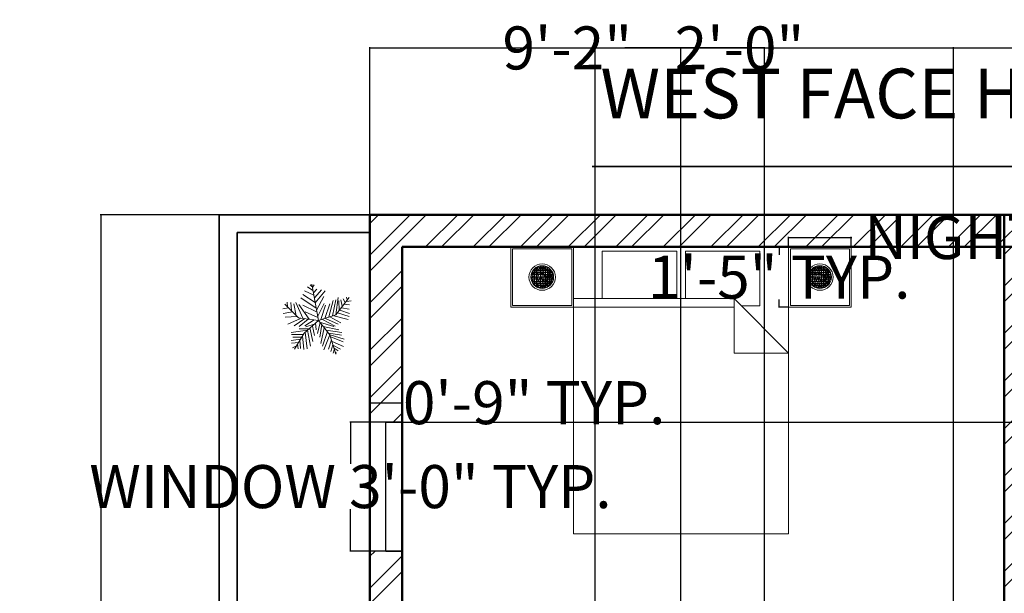
# Model space of a CAD drawing. Units: inches. Extents: x -40 to 578, y -482 to 237.
# Tile 5 of 7: x -26 to 249, y 67 to 227. Entities that reach past the tile are written whole.
import ezdxf

# ---------------------------------------------------------------- set-up
doc = ezdxf.new("R2010")
doc.units = ezdxf.units.IN
doc.header["$MEASUREMENT"] = 0
for name, color, linetype, lineweight in [('A-ANNO-DIMS', 2, 'Continuous', 18), ('A-ANNO-TEXT', 7, 'Continuous', 35), ('A-FURN', 4, 'Continuous', 18), ('A-WALL-PATT', 252, 'Continuous', 13), ('C-PROP', 3, 'Continuous', 35), ('L-PLNT', 94, 'Continuous', 13), ('WALLS', 3, 'Continuous', 50), ('WINDOWS', 241, 'Continuous', 25)]:
    doc.layers.add(name, color=color, linetype=linetype, lineweight=lineweight)
doc.styles.get("Standard").update_dxf_attribs({"font": 'arial.ttf'})
doc.dimstyles.get("Standard").update_dxf_attribs({"dimtxt": 12, "dimasz": 0.18, "dimexe": 0.18, "dimexo": 0.0625, "dimgap": 0.09, "dimtad": 0, "dimtih": 1, "dimtoh": 1, "dimdec": 0, "dimzin": 0, "dimdsep": 46, "dimlunit": 3, "dimtxsty": 'Standard', "dimcen": 0.09, "dimadec": 0, "dimazin": 0, "dimtfac": 1, "dimtdec": 0, "dimtofl": 0, "dimtmove": 0, "dimatfit": 3, "dimfxl": 1, "dimtolj": 1, "dimtzin": 0, "dimarcsym": 0})

# ---------------------------------------------------------------- blocks, each defined once
blk = doc.blocks.new('Bed - Queen')
for p, q in [((0, -80.00003), (0, 0)), ((0, 0), (59.99999, 0)), ((59.99999, 0), (59.99999, -80.00003)), ((7.99999, -1.2), (28.79998, -1.2)), ((7.99999, -14.4), (7.99999, -1.2)), ((28.79998, -1.2), (28.79998, -14.4)), ((31.19999, -1.2), (51.99999, -1.2)), ((31.19999, -14.4), (31.19999, -1.2)), ((51.99999, -1.2), (51.99999, -16.4)), ((0, -14.4), (44.8, -14.4)), ((59.99999, -29.6), (44.8, -14.4)), ((44.8, -14.4), (44.8, -29.6)), ((51.99999, -16.4), (46.79936, -16.4)), ((44.8, -16.8), (0, -16.8)), ((44.8, -29.6), (59.99999, -29.6)), ((59.99999, -80.00003), (0, -80.00003))]:
    blk.add_line(p, q)
blk = doc.blocks.new('*U14')
for p, q in [((-185.1152, 1008.5578), (-553.1612, 1185.4942)), ((-221.9198, 1197.3052), (-433.5526, 1338.8594)), ((-258.7244, 1362.456), (-332.3336, 1421.4348)), ((0, 0), (-266.7, 1447.8)), ((-231.1146, 1315.2628), (-166.7002, 1421.4348)), ((-194.31, 1102.9442), (-65.4812, 1256.284)), ((-148.3106, 914.1968), (118.5418, 1220.9018)), ((-129.8956, 701.8528), (265.7602, 1185.4942)), ((-93.091, 489.5342), (-700.3796, 902.3858)), ((-129.8956, 713.6638), (-626.7704, 1032.1544)), ((-74.7014, 418.7444), (219.7608, 961.39)), ((412.9786, 147.447), (587.8068, 796.2392)), ((560.197, 182.8292), (698.2206, 819.8358)), ((685.8, 228.6), (1219.2, 914.4)), ((689.0258, 230.0224), (790.2448, 914.1968)), ((891.4384, 831.6214), (946.658, 572.1096)), ((983.4626, 867.0036), (1066.2666, 725.4494)), ((1121.4862, 925.9824), (1149.0706, 831.6214)), ((-1206.4492, 501.3198), (-1418.082, 465.9376)), ((-800.1, 114.3), (-1333.5, 647.7)), ((-1234.059, 536.7274), (-1252.4486, 737.2604)), ((-1105.2302, 725.4494), (-1077.6458, 395.1732)), ((-976.4268, 666.4706), (-884.4026, 194.6402)), ((-902.8176, 713.6638), (-617.5756, 100.2538)), ((-369.1382, 53.086), (-783.1836, 642.874)), ((-617.5756, 607.4918), (-74.7014, 347.98)), ((-28.6766, 171.0436), (228.9556, 678.2816)), ((100.1268, 41.275), (284.1498, 619.2774)), ((256.5654, 88.4682), (449.7832, 666.4706)), ((808.6344, 784.4282), (827.0494, 418.7444)), ((845.439, 418.7444), (1241.0948, 277.1902)), ((919.0482, 501.3198), (1222.6798, 454.152)), ((1029.462, 654.685), (1241.0948, 631.0884)), ((1112.2914, 760.8316), (1296.3144, 784.4282)), ((-1031.621, 347.98), (-1399.667, 277.1902)), ((-847.598, 159.2326), (-1326.0578, 135.636)), ((-718.7946, 88.4682), (-1215.644, -147.447)), ((-543.9664, 76.6572), (-967.2066, -206.4512)), ((0, 0), (-800.1, 114.3)), ((-405.9428, 53.086), (-764.794, -241.8334)), ((0, 0), (-571.5, -495.3)), ((-166.7002, 29.4894), (-543.9664, -206.4512)), ((-525.5514, 347.98), (-28.6766, 123.8504)), ((0, 0), (685.8, 228.6)), ((0, 0), (457.2, -571.5)), ((164.5412, 41.275), (661.416, -218.2368)), ((284.1498, 88.4682), (781.0246, -147.447)), ((458.978, 147.447), (891.4384, -88.4682)), ((615.4166, 194.6402), (1185.8752, 41.275)), ((753.4148, 312.5978), (1222.6798, 159.2326)), ((-442.7474, -383.3876), (-1086.8406, -477.7486)), ((-387.5278, -324.4088), (-764.794, -324.4088)), ((-166.7002, -147.447), (-507.1618, -253.619)), ((-433.5526, -383.3876), (-323.1134, -1020.3688)), ((-341.5284, -289.0012), (-221.9198, -831.6214)), ((-240.3094, -218.2368), (-157.5054, -595.7062)), ((-120.7008, -88.4682), (-93.091, -371.5766)), ((63.3222, -76.6826), (-37.8714, -513.1308)), ((44.9326, -64.897), (615.4166, -241.8334)), ((127.7366, -159.258), (54.1274, -654.685)), ((228.9556, -289.0012), (90.932, -914.1968)), ((192.151, -230.0224), (817.8292, -371.5766)), ((311.7596, -383.3876), (937.4378, -477.7486)), ((-718.7946, -737.2604), (-1086.8406, -796.2392)), ((-617.5756, -548.5384), (-1077.6458, -560.324)), ((-681.9646, -666.496), (-1022.4262, -654.685)), ((-571.5, -495.3), (-952.5, -1143)), ((-737.1842, -784.4536), (-709.5744, -1114.7298)), ((-635.9652, -607.5172), (-580.771, -1150.1374)), ((-525.5514, -465.963), (-451.9422, -1126.5408)), ((357.759, -430.5554), (164.5412, -1020.3688)), ((458.978, -572.1096), (210.5406, -1161.923)), ((514.1976, -772.6426), (403.7838, -1138.3264)), ((412.9786, -501.3452), (919.0482, -583.9206)), ((457.2, -571.5), (685.8, -1333.5)), ((468.1982, -572.1096), (1029.462, -737.2604)), ((486.5878, -642.8994), (983.4626, -843.4324)), ((-783.1836, -867.029), (-1077.6458, -902.4112)), ((-875.2078, -1008.5832), (-1040.8412, -1079.3476)), ((-829.2084, -937.7934), (-810.7934, -1126.5408)), ((578.612, -961.39), (495.7826, -1232.7128)), ((541.8074, -831.6214), (992.6574, -1032.1544)), ((578.612, -973.1756), (873.0488, -1138.3264)), ((624.6114, -1161.923), (587.8068, -1291.6916)), ((624.6114, -1102.9442), (781.0246, -1209.1162)), ((679.8056, -1268.095), (716.6102, -1291.6916))]:
    blk.add_line(p, q)
blk = doc.blocks.new('NIGHTSTAND-LAMP')
for p, q in [((7.17, 11.17), (5.64, 7.78)), ((7.58, 11.36), (5.82, 7.16)), ((8.24, 11.54), (6.14, 6.59)), ((8.75, 11.58), (6.65, 6.01)), ((9.21, 11.55), (7.17, 5.63)), ((7.17, 11.17), (10.32, 11.17)), ((7.17, 11.17), (7.17, 5.63)), ((9.71, 11.43), (7.58, 5.44)), ((7.58, 11.36), (7.58, 5.44)), ((8.24, 11.54), (8.24, 5.18)), ((10.22, 11.22), (8.24, 5.26)), ((8.75, 11.58), (8.75, 5.22)), ((9.21, 11.55), (9.21, 5.18)), ((9.71, 11.43), (9.71, 5.37)), ((10.22, 11.22), (10.22, 5.58)), ((6.65, 10.79), (5.56, 8.46)), ((5.56, 8.4), (11.93, 8.4)), ((6.14, 10.22), (5.64, 9.09)), ((5.64, 9.09), (11.85, 9.09)), ((5.64, 9.09), (5.64, 7.71)), ((5.83, 9.68), (11.66, 9.68)), ((6.14, 10.22), (11.36, 10.22)), ((6.14, 10.22), (6.14, 6.58)), ((6.5, 10.65), (10.99, 10.65)), ((6.65, 10.79), (6.65, 6.01)), ((10.75, 10.87), (8.75, 5.22)), ((10.99, 10.65), (9.21, 5.18)), ((11.15, 10.48), (9.71, 5.37)), ((11.36, 10.22), (10.22, 5.58)), ((10.75, 10.87), (10.75, 5.93)), ((11.66, 9.68), (10.75, 5.93)), ((11.15, 10.48), (11.15, 6.31)), ((11.85, 9.09), (11.15, 6.31)), ((11.81, 9.26), (11.81, 7.54)), ((5.63, 7.78), (11.87, 7.78)), ((5.82, 7.16), (11.68, 7.16)), ((6.13, 6.59), (11.37, 6.59)), ((6.6, 6.05), (10.9, 6.05)), ((7.18, 5.63), (10.31, 5.63))]:
    blk.add_line(p, q)
for points in [[(17.49, 16.8), (0, 16.8), (0, 0), (17.49, 0)], [(16.99, 16.3), (0.5, 16.3), (0.5, 0.5), (16.99, 0.5)]]:
    blk.add_lwpolyline(points, close=True)
for radius in [3.68, 3.18]:
    blk.add_circle((8.75, 8.4), radius)
blk = doc.blocks.new('WIN-36IN')
for p, q in [((9, 36), (0, 36)), ((4.5, 0), (4.5, 36)), ((4.5, 36), (9, 36)), ((9, 0), (0, 0)), ((4.5, 0), (9, 0))]:
    blk.add_line(p, q)
blk = doc.blocks.new('*D26')
at = {"layer": 'A-ANNO-DIMS', "color": 0, "lineweight": -2, "transparency": 16777216}
for p, q in [((71.68, 114.63), (66.16, 114.63)), ((66.34, 114.45), (66.34, 102.94)), ((66.34, 78.81), (66.34, 90.33)), ((71.68, 78.63), (66.16, 78.63))]:
    blk.add_line(p, q, dxfattribs=at)
at = {"layer": 'A-ANNO-DIMS', "color": 0, "transparency": 16777216}
for points in [[(66.31, 114.45), (66.37, 114.45), (66.34, 114.63)], [(66.31, 78.81), (66.37, 78.81), (66.34, 78.63)]]:
    blk.add_solid(points, dxfattribs=at)
at = {"layer": 'Defpoints', "color": 0, "transparency": 16777216}
for p in [(66.34, 114.63), (71.74, 114.63), (71.74, 78.63)]:
    blk.add_point(p, dxfattribs=at)
at = {"layer": 'A-ANNO-DIMS', "color": 0, "transparency": 16777216, "insert": (66.34, 96.63), "char_height": 12, "attachment_point": 5}
blk.add_mtext('\\A1;WINDOW 3\'-0" TYP.', dxfattribs=at)
blk = doc.blocks.new('*D27')
at = {"layer": 'A-ANNO-DIMS', "color": 0, "lineweight": -2, "transparency": 16777216}
for p, q in [((71.74, 114.7), (71.74, 120.21)), ((71.92, 120.03), (80.56, 120.03)), ((80.74, 114.7), (80.74, 120.21)), ((80.74, 120.03), (80.92, 120.03))]:
    blk.add_line(p, q, dxfattribs=at)
at = {"layer": 'A-ANNO-DIMS', "color": 0, "transparency": 16777216}
for points in [[(71.92, 120.06), (71.92, 120), (71.74, 120.03)], [(80.56, 120.06), (80.56, 120), (80.74, 120.03)]]:
    blk.add_solid(points, dxfattribs=at)
at = {"layer": 'Defpoints', "color": 0, "transparency": 16777216}
for p in [(80.74, 120.03), (71.74, 114.63), (80.74, 114.63)]:
    blk.add_point(p, dxfattribs=at)
at = {"layer": 'A-ANNO-DIMS', "color": 0, "transparency": 16777216, "insert": (117.58, 120.03), "char_height": 12, "attachment_point": 5}
blk.add_mtext('\\A1;0\'-9" TYP.', dxfattribs=at)
blk = doc.blocks.new('*D28')
at = {"layer": 'A-ANNO-DIMS', "color": 0, "lineweight": -2, "transparency": 16777216}
for p, q in [((188.56, 163.51), (188.56, 166.25)), ((188.74, 166.07), (205.87, 166.07)), ((206.05, 163.51), (206.05, 166.25)), ((206.05, 166.07), (206.23, 166.07))]:
    blk.add_line(p, q, dxfattribs=at)
at = {"layer": 'A-ANNO-DIMS', "color": 0, "transparency": 16777216}
for points in [[(188.74, 166.1), (188.74, 166.04), (188.56, 166.07)], [(205.87, 166.1), (205.87, 166.04), (206.05, 166.07)]]:
    blk.add_solid(points, dxfattribs=at)
at = {"layer": 'Defpoints', "color": 0, "transparency": 16777216}
for p in [(206.05, 166.07), (188.56, 163.45), (206.05, 163.45)]:
    blk.add_point(p, dxfattribs=at)
at = {"layer": 'A-ANNO-DIMS', "color": 0, "transparency": 16777216, "insert": (313.4, 166.07), "char_height": 12, "attachment_point": 5}
blk.add_mtext('\\A1;NIGHTSTAND 1\'-5 1/2" TYP.', dxfattribs=at)
blk = doc.blocks.new('*D29')
at = {"layer": 'A-ANNO-DIMS', "color": 0, "lineweight": -2, "transparency": 16777216}
for p, q in [((188.5, 163.45), (185.76, 163.45)), ((185.94, 163.27), (185.94, 161.26)), ((185.94, 146.83), (185.94, 148.83)), ((188.5, 146.65), (185.76, 146.65))]:
    blk.add_line(p, q, dxfattribs=at)
at = {"layer": 'A-ANNO-DIMS', "color": 0, "transparency": 16777216}
for points in [[(185.91, 163.27), (185.97, 163.27), (185.94, 163.45)], [(185.91, 146.83), (185.97, 146.83), (185.94, 146.65)]]:
    blk.add_solid(points, dxfattribs=at)
at = {"layer": 'Defpoints', "color": 0, "transparency": 16777216}
for p in [(185.94, 163.45), (188.56, 163.45), (188.56, 146.65)]:
    blk.add_point(p, dxfattribs=at)
at = {"layer": 'A-ANNO-DIMS', "color": 0, "transparency": 16777216, "insert": (185.94, 155.05), "char_height": 12, "attachment_point": 5}
blk.add_mtext('\\A1;1\'-5" TYP.', dxfattribs=at)
blk = doc.blocks.new('*D42')
at = {"layer": 'A-ANNO-DIMS', "color": 0, "lineweight": -2, "transparency": 16777216}
for p, q in [((71.78, -441.49), (71.78, 219.12)), ((71.96, 218.94), (110.77, 218.94)), ((181.65, 218.94), (142.84, 218.94)), ((181.83, -441.49), (181.83, 219.12))]:
    blk.add_line(p, q, dxfattribs=at)
at = {"layer": 'A-ANNO-DIMS', "color": 0, "transparency": 16777216}
for points in [[(71.96, 218.97), (71.96, 218.91), (71.78, 218.94)], [(181.65, 218.97), (181.65, 218.91), (181.83, 218.94)]]:
    blk.add_solid(points, dxfattribs=at)
at = {"layer": 'Defpoints', "color": 0, "transparency": 16777216}
for p in [(181.83, 218.94), (71.78, -441.55), (181.83, -441.55)]:
    blk.add_point(p, dxfattribs=at)
at = {"layer": 'A-ANNO-DIMS', "color": 0, "transparency": 16777216, "insert": (126.81, 218.94), "char_height": 12, "attachment_point": 5}
blk.add_mtext('\\A1;9\'-2"', dxfattribs=at)
blk = doc.blocks.new('*D44')
at = {"layer": 'A-ANNO-DIMS', "color": 0, "lineweight": -2, "transparency": 16777216}
for p, q in [((29.68, 172.45), (-3.49, 172.45)), ((-3.31, 172.27), (-3.31, -128.34)), ((-3.31, -441.37), (-3.31, -140.77)), ((29.68, -441.55), (-3.49, -441.55))]:
    blk.add_line(p, q, dxfattribs=at)
at = {"layer": 'A-ANNO-DIMS', "color": 0, "transparency": 16777216}
for points in [[(-3.34, 172.27), (-3.28, 172.27), (-3.31, 172.45)], [(-3.34, -441.37), (-3.28, -441.37), (-3.31, -441.55)]]:
    blk.add_solid(points, dxfattribs=at)
at = {"layer": 'Defpoints', "color": 0, "transparency": 16777216}
for p in [(-3.31, 172.45), (29.74, 172.45), (29.74, -441.55)]:
    blk.add_point(p, dxfattribs=at)
at = {"layer": 'A-ANNO-DIMS', "color": 0, "transparency": 16777216, "insert": (-3.31, -134.55), "char_height": 12, "attachment_point": 5}
blk.add_mtext('\\A1;51\'-2"', dxfattribs=at)
blk = doc.blocks.new('*D45')
at = {"layer": 'A-ANNO-DIMS', "color": 0, "lineweight": -2, "transparency": 16777216}
for p, q in [((71.74, 172.51), (71.74, 219.12)), ((71.92, 218.94), (257.04, 218.94)), ((483.56, 218.94), (298.43, 218.94)), ((483.74, 172.51), (483.74, 219.12))]:
    blk.add_line(p, q, dxfattribs=at)
at = {"layer": 'A-ANNO-DIMS', "color": 0, "transparency": 16777216}
for points in [[(71.92, 218.97), (71.92, 218.91), (71.74, 218.94)], [(483.56, 218.97), (483.56, 218.91), (483.74, 218.94)]]:
    blk.add_solid(points, dxfattribs=at)
at = {"layer": 'Defpoints', "color": 0, "transparency": 16777216}
for p in [(483.74, 218.94), (71.74, 172.45), (483.74, 172.45)]:
    blk.add_point(p, dxfattribs=at)
at = {"layer": 'A-ANNO-DIMS', "color": 0, "transparency": 16777216, "insert": (277.74, 218.94), "char_height": 12, "attachment_point": 5}
blk.add_mtext('\\A1;34\'-4"', dxfattribs=at)
blk = doc.blocks.new('*D52')
at = {"layer": 'A-ANNO-DIMS', "color": 0, "lineweight": -2, "transparency": 16777216}
for p, q in [((234.57, -377.49), (234.57, 219.12)), ((234.75, 218.94), (265.48, 218.94)), ((265.66, -377.49), (265.66, 219.12)), ((265.66, 218.94), (265.84, 218.94))]:
    blk.add_line(p, q, dxfattribs=at)
at = {"layer": 'A-ANNO-DIMS', "color": 0, "transparency": 16777216}
for points in [[(234.75, 218.97), (234.75, 218.91), (234.57, 218.94)], [(265.48, 218.97), (265.48, 218.91), (265.66, 218.94)]]:
    blk.add_solid(points, dxfattribs=at)
at = {"layer": 'Defpoints', "color": 0, "transparency": 16777216}
for p in [(265.66, 218.94), (234.57, -377.55), (265.66, -377.55)]:
    blk.add_point(p, dxfattribs=at)
at = {"layer": 'A-ANNO-DIMS', "color": 0, "transparency": 16777216, "insert": (281.98, 218.94), "char_height": 12, "attachment_point": 5}
blk.add_mtext('\\A1;2\'-7"', dxfattribs=at)
blk = doc.blocks.new('*D55')
at = {"layer": 'A-ANNO-DIMS', "color": 0, "lineweight": -2, "transparency": 16777216}
for p, q in [((134.6, 25.51), (134.6, 219.12)), ((134.78, 218.94), (158.35, 218.94)), ((158.53, 25.51), (158.53, 219.12)), ((158.53, 218.94), (158.71, 218.94))]:
    blk.add_line(p, q, dxfattribs=at)
at = {"layer": 'A-ANNO-DIMS', "color": 0, "transparency": 16777216}
for points in [[(134.78, 218.97), (134.78, 218.91), (134.6, 218.94)], [(158.35, 218.97), (158.35, 218.91), (158.53, 218.94)]]:
    blk.add_solid(points, dxfattribs=at)
at = {"layer": 'Defpoints', "color": 0, "transparency": 16777216}
for p in [(158.53, 218.94), (134.6, 25.45), (158.53, 25.45)]:
    blk.add_point(p, dxfattribs=at)
at = {"layer": 'A-ANNO-DIMS', "color": 0, "transparency": 16777216, "insert": (174.86, 218.94), "char_height": 12, "attachment_point": 5}
blk.add_mtext('\\A1;2\'-0"', dxfattribs=at)
blk = doc.blocks.new('*D62')
at = {"layer": 'A-ANNO-DIMS', "color": 0, "lineweight": -2, "transparency": 16777216}
for p, q in [((80.8, 163.45), (516.97, 163.45)), ((516.79, 163.27), (516.79, 145.16)), ((516.79, 114.81), (516.79, 132.93)), ((80.8, 114.63), (516.97, 114.63))]:
    blk.add_line(p, q, dxfattribs=at)
at = {"layer": 'A-ANNO-DIMS', "color": 0, "transparency": 16777216}
for points in [[(516.76, 163.27), (516.82, 163.27), (516.79, 163.45)], [(516.76, 114.81), (516.82, 114.81), (516.79, 114.63)]]:
    blk.add_solid(points, dxfattribs=at)
at = {"layer": 'Defpoints', "color": 0, "transparency": 16777216}
for p in [(80.74, 163.45), (80.74, 114.63), (516.79, 114.63)]:
    blk.add_point(p, dxfattribs=at)
at = {"layer": 'A-ANNO-DIMS', "color": 0, "transparency": 16777216, "insert": (516.79, 139.04), "char_height": 12, "attachment_point": 5}
blk.add_mtext('\\A1;4\'-1"', dxfattribs=at)

msp = doc.modelspace()

# ---------------------------------------------------------------- hatches: boundary and pattern name
at = {"layer": 'A-WALL-PATT'}
h = msp.add_hatch(dxfattribs=at)
h.set_pattern_fill('ANSI32', color=256, scale=25)
h.set_pattern_definition([(45, (-1993.713, -1175.095), (-6.629126, 6.629126), []), (45, (-1989.294, -1175.095), (-6.629126, 6.629126), [])])
h.paths.add_polyline_path([(248.74, 172.45), (71.74, 172.45), (71.74, 114.63), (80.74, 114.63), (80.74, 163.45), (248.74, 163.45)])
h.paths.add_polyline_path([(253.74, 172.45), (248.74, 172.45), (248.74, 163.45), (253.74, 163.45)])
h.paths.add_polyline_path([(253.74, 163.45), (248.74, 163.45), (248.74, 25.45), (240.62, 25.45), (240.62, 20.45), (263.71, 20.45), (263.71, 25.45), (253.74, 25.45)])
h.paths.add_polyline_path([(483.74, 172.45), (253.74, 172.45), (253.74, 163.45), (426.74, 163.45), (474.74, 163.45), (474.74, 79.45), (465.23, 79.45), (465.23, 77.2), (441.23, 77.2), (441.23, 74.45), (483.74, 74.45)])
h.paths.add_polyline_path([(80.74, 78.63), (71.74, 78.63), (71.74, 3.32), (80.74, 3.32), (80.74, 20.45), (134.6, 20.45), (134.6, 25.45), (80.74, 25.45)])
h.paths.add_polyline_path([(202.4, 25.45), (158.53, 25.45), (158.53, 20.45), (202.4, 20.45)])
h.paths.add_polyline_path([(169.74, 20.45), (164.74, 20.45), (164.74, -39.55), (80.74, -39.55), (80.74, -20.68), (71.74, -20.68), (71.74, -61.38), (80.74, -61.38), (80.74, -44.55), (164.74, -44.55), (164.74, -104.55), (169.74, -104.55), (169.74, -44.55)])
h.paths.add_polyline_path([(135.96, -104.55), (80.74, -104.55), (80.74, -85.38), (71.74, -85.38), (71.74, -155.89), (80.74, -155.89), (80.74, -109.55), (135.96, -109.55)])
h.paths.add_polyline_path([(218.74, -104.55), (159.9, -104.55), (159.9, -109.55), (218.74, -109.55)])
h.paths.add_polyline_path([(223.74, -104.55), (218.74, -104.55), (218.74, -109.55), (223.74, -109.55)])
h.paths.add_polyline_path([(223.74, -109.55), (218.74, -109.55), (218.74, -114.58), (223.74, -114.58)])
h.paths.add_polyline_path([(430.74, -85.66), (421.74, -85.66), (421.74, -128.55), (223.74, -128.55), (223.74, -133.55), (421.74, -133.55), (421.74, -197.77), (430.74, -197.77)])
h.paths.add_polyline_path([(223.74, -152.8), (218.74, -152.8), (218.74, -229.55), (151.59, -229.55), (151.59, -238.55), (223.74, -238.55), (223.74, -229.55)])
h.paths.add_polyline_path([(115.59, -229.55), (98.23, -229.55), (80.74, -229.55), (80.74, -212.75), (80.74, -191.89), (71.74, -191.89), (71.74, -238.55), (115.59, -238.55)])
h.paths.add_polyline_path([(307.53, -289.55), (223.74, -289.55), (223.74, -283.47), (218.74, -283.47), (218.74, -298.55), (307.53, -298.55)])
h.paths.add_polyline_path([(421.74, -289.55), (343.53, -289.55), (343.53, -298.55), (421.74, -298.55)])
h.paths.add_polyline_path([(430.74, -367.34), (421.74, -367.34), (421.74, -377.55), (234.57, -377.55), (234.57, -386.55), (430.74, -386.55)])
h.paths.add_polyline_path([(430.74, -298.55), (430.74, -233.77), (421.74, -233.77), (421.74, -289.55), (421.74, -298.55), (421.74, -331.34), (430.74, -331.34)])
h.paths.add_polyline_path([(430.74, -11.67), (427.15, -11.67, -0.057068), (421.74, -11.05), (421.74, -49.66), (430.74, -49.66)])
h.paths.add_polyline_path([(430.74, 31.9), (421.74, 31.9), (421.74, 25.45), (301.93, 25.45), (301.93, 20.45), (421.74, 20.45), (421.74, 12.26), (430.74, 12.26)])
h.paths.add_polyline_path([(426.74, 134.23, -0.014739), (425.33, 134.19), (421.74, 134.19), (421.74, 74.45), (441.23, 74.45), (441.23, 77.2), (441.23, 79.45), (426.74, 79.45)], flags=17)
h.paths.add_polyline_path([(430.74, 74.45), (421.74, 74.45), (421.74, 67.9), (430.74, 67.9)])

# ---------------------------------------------------------------- linework, layer by layer
at = {"layer": 'A-ANNO-TEXT'}
msp.add_line((133.78, 185.89), (385.18, 185.89), dxfattribs=at)
at = {"layer": 'C-PROP'}
for p, q in [((71.74, 172.45), (29.74, 172.45)), ((29.74, 172.45), (29.74, -441.55)), ((71.74, 167.45), (34.74, 167.45)), ((34.74, 167.45), (34.74, -432.55))]:
    msp.add_line(p, q, dxfattribs=at)
at = {"layer": 'WALLS'}
for p, q in [((71.74, 172.45), (71.74, -238.55)), ((483.74, 172.45), (71.74, 172.45)), ((248.74, 172.45), (248.74, 25.45)), ((80.74, 163.45), (80.74, 25.45)), ((426.74, 163.45), (80.74, 163.45))]:
    msp.add_line(p, q, dxfattribs=at)

# ---------------------------------------------------------------- block references
at = {"layer": 'A-FURN'}
for name, p in [('NIGHTSTAND-LAMP', (111.07, 146.65)), ('Bed - Queen', (128.56, 163.45)), ('NIGHTSTAND-LAMP', (188.56, 146.65))]:
    msp.add_blockref(name, p, dxfattribs=at)
at = {"layer": 'L-PLNT', "xscale": 0.0070029080995801, "yscale": 0.0070029080995801, "zscale": 0.0070029080995801}
msp.add_blockref('*U14', (57.41, 142.92), dxfattribs=at)
at = {"layer": 'WINDOWS'}
msp.add_blockref('WIN-36IN', (71.74, 78.64), dxfattribs=at)

# ---------------------------------------------------------------- texts
at = {"layer": 'A-ANNO-TEXT'}
msp.add_text('WEST FACE HOUSE PLAN', height=13.8818, dxfattribs=at).set_placement((136.08, 199.3))

# ---------------------------------------------------------------- dimensions: what is measured, and where the dimension line sits
at = {"layer": 'A-ANNO-DIMS'}
for base, p1, p2, picture, middle in [((483.74, 218.94), (71.74, 172.45), (483.74, 172.45), '*D45', (277.74, 218.94)), ((181.8272, 218.9381), (71.7835, -441.5525), (181.8272, -441.5525), '*D42', (126.8054, 218.9381)), ((158.53, 218.94), (134.6, 25.45), (158.53, 25.45), '*D55', (174.86, 218.94)), ((265.66, 218.94), (234.57, -377.55), (265.66, -377.55), '*D52', (281.98, 218.94))]:
    dim = msp.add_linear_dim(base=base, p1=p1, p2=p2, dimstyle='Standard', override={"dimdec": 1, "dimlfac": 1, "dimrnd": 0, "dimzin": 1, "dimdsep": 46, "dimlunit": 4, "dimfrac": 2}, dxfattribs=at)
    dim.commit()
    dim.dimension.update_dxf_attribs({"geometry": picture, "text_midpoint": middle})
for base, p1, p2, text, picture, middle in [((206.05, 166.07), (188.56, 163.45), (206.05, 163.45), 'NIGHTSTAND <> TYP.', '*D28', (313.4, 166.07)), ((80.74, 120.03), (71.74, 114.63), (80.74, 114.63), '<> TYP.', '*D27', (117.58, 120.03))]:
    dim = msp.add_linear_dim(base=base, p1=p1, p2=p2, text=text, dimstyle='Standard', override={"dimdec": 1, "dimlfac": 1, "dimrnd": 0, "dimzin": 1, "dimdsep": 46, "dimlunit": 4, "dimfrac": 2}, dxfattribs=at)
    dim.commit()
    dim.dimension.update_dxf_attribs({"geometry": picture, "text_midpoint": middle})
for base, p1, p2, picture, middle in [((-3.31, 172.45), (29.74, -441.55), (29.74, 172.45), '*D44', (-3.31, -134.55)), ((516.79, 114.63), (80.74, 163.45), (80.74, 114.63), '*D62', (516.79, 139.04))]:
    dim = msp.add_linear_dim(base=base, p1=p1, p2=p2, angle=90, dimstyle='Standard', override={"dimdec": 1, "dimlfac": 1, "dimrnd": 0, "dimzin": 1, "dimdsep": 46, "dimlunit": 4, "dimfrac": 2}, dxfattribs=at)
    dim.commit()
    dim.dimension.update_dxf_attribs({"geometry": picture, "text_midpoint": middle})
for base, p1, p2, text, picture, middle in [((185.94, 163.45), (188.56, 146.65), (188.56, 163.45), '<> TYP.', '*D29', (185.94, 155.05)), ((66.34, 114.63), (71.74, 78.63), (71.74, 114.63), 'WINDOW <> TYP.', '*D26', (66.34, 96.63))]:
    dim = msp.add_linear_dim(base=base, p1=p1, p2=p2, angle=90, text=text, dimstyle='Standard', override={"dimdec": 1, "dimlfac": 1, "dimrnd": 0, "dimzin": 1, "dimdsep": 46, "dimlunit": 4, "dimfrac": 2}, dxfattribs=at)
    dim.commit()
    dim.dimension.update_dxf_attribs({"geometry": picture, "text_midpoint": middle})

doc.saveas('drawing.dxf')
